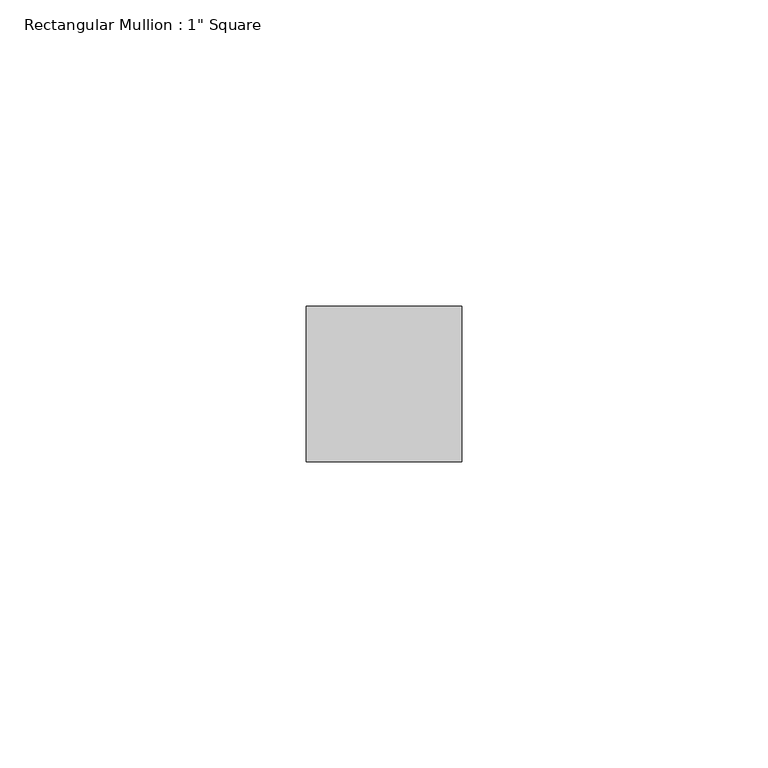
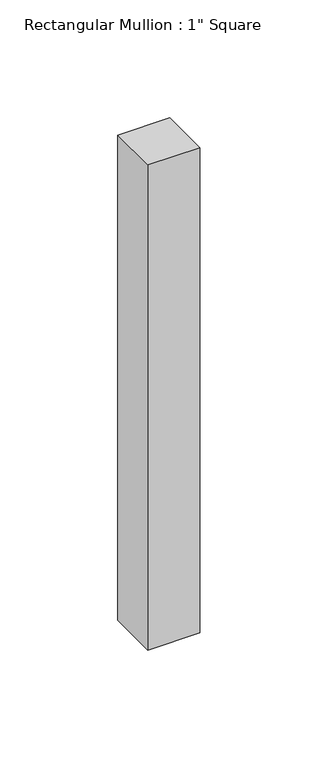
"""IFC4 building model written with IfcOpenShell, lengths in millimetres: member geometry."""

from ifc_helpers import new_model, si_unit, frame, origin, place, context, project, spatial, polyline, outline, extrude, source, transform, mapped, element, save


def member_63f4cac5(model_context):
    return source(origin(), model_context, "Body", "SweptSolid", [
        extrude(outline(polyline([(12.7, 12.7), (12.7, -12.7), (-12.7, -12.7), (-12.7, 12.7), (12.7, 12.7)])), frame((0.0, 0.0, -251.1186703), z_axis=(0.0, 0.0, 1.0), x_axis=(1.0, 0.0, 0.0)), (0.0, 0.0, 1.0), 251.1186703),
    ])


if __name__ == "__main__":
    model = new_model("IFC4")
    model_context = context("Model", 3, world=origin())
    ifc_project = project(units=[si_unit("LENGTHUNIT", "METRE", prefix="MILLI")], contexts=[model_context])
    site = spatial("IfcSite", under=ifc_project)
    building = spatial("IfcBuilding", under=site)
    placement = place(None, origin())
    member_shape = member_63f4cac5(model_context)
    element("IfcMember", 1, ObjectType="Rectangular Mullion : 1\" Square", at=placement, inside=building, context=model_context, shape_type="MappedRepresentation", body=[
        mapped(member_shape, transform((0.0, 0.0, 0.0), x_axis=(1.0, 0.0, 0.0), y_axis=(0.0, 1.0, 0.0), z_axis=(0.0, 0.0, 1.0))),
    ])
    save(model, "model.ifc")

# Revit data of these elements
# Type "Rectangular Mullion : 1\" Square"
#   built-in parameter 1007304 = 0.0833333 (stored number, unit not read)
#   built-in parameter 1007301 = 0.0416667 (stored number, unit not read)
#   built-in parameter 1007300 = 0.0416667 (stored number, unit not read)
